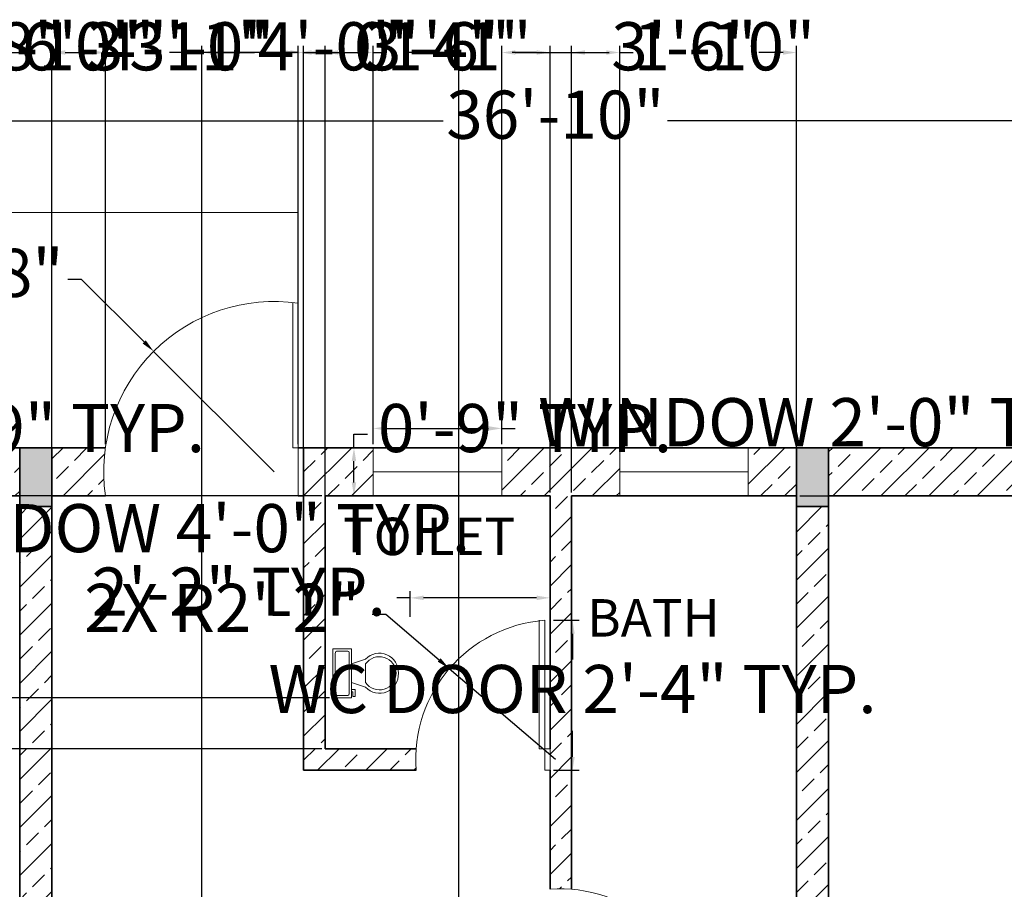
# Model space of a CAD drawing. Units: inches. Extents: x 9689 to 10369, y 10965 to 11626.
# Tile 8 of 11: x 9923 to 10107, y 11456 to 11619. Entities that reach past the tile are written whole.
import ezdxf

# ---------------------------------------------------------------- set-up
doc = ezdxf.new("R2010")
doc.units = ezdxf.units.IN
for name, color, linetype, lineweight in [('A-ANNO-DIMS', 2, 'Continuous', 18), ('A-AREA-IDEN', 7, 'Continuous', 18), ('A-COLS', 7, 'Continuous', 35), ('A-DOOR', 4, 'Continuous', 18), ('A-FLOR-FIXT', 8, 'Continuous', 18), ('A-FLOR-STRS', 7, 'Continuous', 18), ('A-GLAZ', 4, 'Continuous', 18), ('A-WALL', 7, 'Continuous', 35), ('A-WALL-PATT', 252, 'Continuous', 13)]:
    doc.layers.add(name, color=color, linetype=linetype, lineweight=lineweight)
doc.layers.add('A-COLS-PATT', color=18, linetype='Continuous', lineweight=13, true_color=0x000000)
doc.styles.get("Standard").update_dxf_attribs({"font": 'arial.ttf'})
doc.dimstyles.new('ISO-25', dxfattribs={"dimtxt": 9, "dimasz": 2.5, "dimexe": 1.25, "dimexo": 0.625, "dimgap": 2, "dimtad": 0, "dimtih": 1, "dimtoh": 1, "dimdec": 1, "dimlunit": 4, "dimtxsty": 'Standard', "dimcen": 2.5, "dimadec": 0, "dimazin": 0, "dimtfac": 0.5, "dimtdec": 1, "dimtmove": 0, "dimatfit": 3, "dimfxl": 1, "dimarcsym": 0})

# ---------------------------------------------------------------- blocks, each defined once
blk = doc.blocks.new('*U16')
for p, q in [((241.3, -152.4), (241.3, -50.8)), ((-203.2, -215.9), (-203.2, -203.2)), ((-177.8, -203.2), (-177.8, -241.3)), ((-101.6, -203.2), (-152.4, -355.6)), ((101.6, -203.2), (152.4, -355.6)), ((-254, -215.9), (-203.2, -215.9)), ((-254, -241.3), (-254, -215.9)), ((-177.8, -241.3), (-254, -241.3)), ((101.6, -355.6), (-101.6, -355.6))]:
    blk.add_line(p, q)
blk.add_lwpolyline([(266.7, -203.2), (266.7, 0), (-266.7, 0), (-266.7, -203.2)], close=True)
for points in [[(-241.3, -50.8), (-241.3, -152.4)], [(215.9, -25.4), (-215.9, -25.4)], [(-215.9, -177.8), (215.9, -177.8)]]:
    blk.add_lwpolyline(points)
for centre, radius, start, end in [((-219.075, -47.625), 22.45064, 81.8699, 188.1301), ((219.075, -47.625), 22.45064, 351.8699, 98.1301), ((-219.075, -155.575), 22.45064, 171.869898, 278.1301), ((219.075, -155.575), 22.45064, 261.8699, 8.1301), ((-12.12088, -505.93752), 205.61935, 133.01722, 273.38), ((0.94996, -504.77674), 181.02486, 124.50543, 269.7), ((-0.94742, -504.77674), 181.02486, 270.3, 55.4946), ((12.12342, -505.93752), 205.61935, 266.62, 46.9828)]:
    blk.add_arc(centre, radius, start, end)
blk = doc.blocks.new('*D21')
at = {"layer": 'A-ANNO-DIMS', "color": 0, "lineweight": -2, "transparency": 16777216}
for p, q in [((9802.06, 11539.26), (9802.06, 11600.92)), ((10244.06, 11539.26), (10244.06, 11600.92)), ((9804.56, 11599.67), (10002.11, 11599.67)), ((10241.56, 11599.67), (10044.01, 11599.67))]:
    blk.add_line(p, q, dxfattribs=at)
at = {"layer": 'A-ANNO-DIMS', "color": 0, "transparency": 16777216}
for points in [[(9804.56, 11600.08), (9804.56, 11599.25), (9802.06, 11599.67)], [(10241.56, 11600.08), (10241.56, 11599.25), (10244.06, 11599.67)]]:
    blk.add_solid(points, dxfattribs=at)
at = {"layer": 'Defpoints', "color": 0, "transparency": 16777216}
for p in [(10244.06, 11599.67), (9802.06, 11538.63), (10244.06, 11538.63)]:
    blk.add_point(p, dxfattribs=at)
at = {"layer": 'A-ANNO-DIMS', "color": 0, "transparency": 16777216, "insert": (10023.06, 11599.67), "char_height": 9, "attachment_point": 5}
blk.add_mtext('36\'-10"', dxfattribs=at)
blk = doc.blocks.new('WINDOW-24')
for p, q in [((0, 0), (0, 9)), ((24, 0), (24, 9)), ((0, 4.5), (24, 4.5))]:
    blk.add_line(p, q)
blk = doc.blocks.new('DOOR-SWING-24')
for p, q in [((4, 2), (28, 2)), ((4, 2), (4, 0)), ((0, 1), (4, 1)), ((0, 1), (0, 0)), ((0, 0), (4, 0)), ((4, 1), (28, 1))]:
    blk.add_line(p, q)
blk.add_arc((2, -1), 26.08, 4.3987, 94.3987)
blk = doc.blocks.new('*D34')
at = {"layer": 'A-ANNO-DIMS', "color": 0, "lineweight": -2, "transparency": 16777216}
for p, q in [((10022.68, 11506.38), (10027.51, 11506.38)), ((10026.26, 11503.88), (10026.26, 11499.04)), ((10026.26, 11480.88), (10026.26, 11485.72)), ((10022.68, 11478.38), (10027.51, 11478.38))]:
    blk.add_line(p, q, dxfattribs=at)
at = {"layer": 'A-ANNO-DIMS', "color": 0, "transparency": 16777216}
for points in [[(10025.84, 11503.88), (10026.67, 11503.88), (10026.26, 11506.38)], [(10025.84, 11480.88), (10026.67, 11480.88), (10026.26, 11478.38)]]:
    blk.add_solid(points, dxfattribs=at)
at = {"layer": 'Defpoints', "color": 0, "transparency": 16777216}
for p in [(10022.06, 11506.38), (10026.26, 11506.38), (10022.06, 11478.38)]:
    blk.add_point(p, dxfattribs=at)
at = {"layer": 'A-ANNO-DIMS', "color": 0, "transparency": 16777216, "insert": (10026.26, 11492.38), "char_height": 9, "attachment_point": 5}
blk.add_mtext('WC DOOR 2\'-4" TYP.', dxfattribs=at)
blk = doc.blocks.new('*D35')
at = {"layer": 'A-ANNO-DIMS', "color": 0, "lineweight": -2, "transparency": 16777216}
for p, q in [((9995.95, 11507.01), (9995.95, 11511.83)), ((10022.06, 11507.01), (10022.06, 11511.83)), ((9995.95, 11510.58), (9993.45, 11510.58)), ((10019.56, 11510.58), (9998.45, 11510.58))]:
    blk.add_line(p, q, dxfattribs=at)
at = {"layer": 'A-ANNO-DIMS', "color": 0, "transparency": 16777216}
for points in [[(9998.45, 11511), (9998.45, 11510.16), (9995.95, 11510.58)], [(10019.56, 11511), (10019.56, 11510.16), (10022.06, 11510.58)]]:
    blk.add_solid(points, dxfattribs=at)
at = {"layer": 'Defpoints', "color": 0, "transparency": 16777216}
for p in [(9995.95, 11510.58), (9995.95, 11506.38), (10022.06, 11506.38)]:
    blk.add_point(p, dxfattribs=at)
at = {"layer": 'A-ANNO-DIMS', "color": 0, "transparency": 16777216, "insert": (9963.95, 11510.58), "char_height": 9, "attachment_point": 5}
blk.add_mtext('2\'-2" TYP.', dxfattribs=at)
blk = doc.blocks.new('*D42')
at = {"layer": 'A-ANNO-DIMS', "color": 0, "lineweight": -2, "transparency": 16777216}
for p, q in [((9843.06, 11529.01), (9843.06, 11521.18)), ((9891.06, 11529.01), (9891.06, 11521.18)), ((9845.56, 11522.43), (9888.56, 11522.43)), ((9891.06, 11522.43), (9893.56, 11522.43))]:
    blk.add_line(p, q, dxfattribs=at)
at = {"layer": 'A-ANNO-DIMS', "color": 0, "transparency": 16777216}
for points in [[(9845.56, 11522.85), (9845.56, 11522.01), (9843.06, 11522.43)], [(9888.56, 11522.85), (9888.56, 11522.01), (9891.06, 11522.43)]]:
    blk.add_solid(points, dxfattribs=at)
at = {"layer": 'Defpoints', "color": 0, "transparency": 16777216}
for p in [(9843.06, 11529.63), (9891.06, 11529.63), (9891.06, 11522.43)]:
    blk.add_point(p, dxfattribs=at)
at = {"layer": 'A-ANNO-DIMS', "color": 0, "transparency": 16777216, "insert": (9952.5, 11522.43), "char_height": 9, "attachment_point": 5}
blk.add_mtext('WINDOW 4\'-0" TYP.', dxfattribs=at)
blk = doc.blocks.new('*D43')
at = {"layer": 'A-ANNO-DIMS', "color": 0, "lineweight": -2, "transparency": 16777216}
for p, q in [((9898.26, 11538.63), (9898.26, 11541.13)), ((9898.26, 11541.13), (9900.76, 11541.13)), ((9891.68, 11538.63), (9899.51, 11538.63)), ((9898.26, 11532.13), (9898.26, 11536.13)), ((9891.68, 11529.63), (9899.51, 11529.63))]:
    blk.add_line(p, q, dxfattribs=at)
at = {"layer": 'A-ANNO-DIMS', "color": 0, "transparency": 16777216}
for points in [[(9897.84, 11536.13), (9898.67, 11536.13), (9898.26, 11538.63)], [(9897.84, 11532.13), (9898.67, 11532.13), (9898.26, 11529.63)]]:
    blk.add_solid(points, dxfattribs=at)
at = {"layer": 'Defpoints', "color": 0, "transparency": 16777216}
for p in [(9891.06, 11538.63), (9898.26, 11538.63), (9891.06, 11529.63)]:
    blk.add_point(p, dxfattribs=at)
at = {"layer": 'A-ANNO-DIMS', "color": 0, "transparency": 16777216, "insert": (9930.19, 11541.13), "char_height": 9, "attachment_point": 5}
blk.add_mtext('0\'-9" TYP.', dxfattribs=at)
blk = doc.blocks.new('*D44')
at = {"layer": 'A-ANNO-DIMS', "color": 0, "lineweight": -2, "transparency": 16777216}
for p, q in [((9989.06, 11539.26), (9989.06, 11543.48)), ((10013.06, 11539.26), (10013.06, 11543.48)), ((9991.56, 11542.23), (10010.56, 11542.23)), ((10013.06, 11542.23), (10015.56, 11542.23))]:
    blk.add_line(p, q, dxfattribs=at)
at = {"layer": 'A-ANNO-DIMS', "color": 0, "transparency": 16777216}
for points in [[(9991.56, 11542.65), (9991.56, 11541.81), (9989.06, 11542.23)], [(10010.56, 11542.65), (10010.56, 11541.81), (10013.06, 11542.23)]]:
    blk.add_solid(points, dxfattribs=at)
at = {"layer": 'Defpoints', "color": 0, "transparency": 16777216}
for p in [(10013.06, 11542.23), (9989.06, 11538.63), (10013.06, 11538.63)]:
    blk.add_point(p, dxfattribs=at)
at = {"layer": 'A-ANNO-DIMS', "color": 0, "transparency": 16777216, "insert": (10074.5, 11542.23), "char_height": 9, "attachment_point": 5}
blk.add_mtext('WINDOW 2\'-0" TYP.', dxfattribs=at)
blk = doc.blocks.new('*D45')
at = {"layer": 'A-ANNO-DIMS', "color": 0, "lineweight": -2, "transparency": 16777216}
for p, q in [((9985.46, 11538.63), (9985.46, 11541.13)), ((9985.46, 11541.13), (9987.96, 11541.13)), ((9988.43, 11538.63), (9984.21, 11538.63)), ((9985.46, 11532.13), (9985.46, 11536.13)), ((9988.43, 11529.63), (9984.21, 11529.63))]:
    blk.add_line(p, q, dxfattribs=at)
at = {"layer": 'A-ANNO-DIMS', "color": 0, "transparency": 16777216}
for points in [[(9985.04, 11536.13), (9985.87, 11536.13), (9985.46, 11538.63)], [(9985.04, 11532.13), (9985.87, 11532.13), (9985.46, 11529.63)]]:
    blk.add_solid(points, dxfattribs=at)
at = {"layer": 'Defpoints', "color": 0, "transparency": 16777216}
for p in [(9985.46, 11538.63), (9989.06, 11538.63), (9989.06, 11529.63)]:
    blk.add_point(p, dxfattribs=at)
at = {"layer": 'A-ANNO-DIMS', "color": 0, "transparency": 16777216, "insert": (10017.39, 11541.13), "char_height": 9, "attachment_point": 5}
blk.add_mtext('0\'-9" TYP.', dxfattribs=at)
blk = doc.blocks.new('*D78')
at = {"layer": 'A-ANNO-DIMS', "color": 0, "lineweight": -2, "transparency": 16777216}
for p, q in [((9980.06, 11530.26), (9980.06, 11613.7)), ((10022.06, 11530.26), (10022.06, 11613.7)), ((9982.56, 11612.45), (9987.1, 11612.45)), ((10019.56, 11612.45), (10015.02, 11612.45))]:
    blk.add_line(p, q, dxfattribs=at)
at = {"layer": 'A-ANNO-DIMS', "color": 0, "transparency": 16777216}
for points in [[(9982.56, 11612.87), (9982.56, 11612.04), (9980.06, 11612.45)], [(10019.56, 11612.87), (10019.56, 11612.04), (10022.06, 11612.45)]]:
    blk.add_solid(points, dxfattribs=at)
at = {"layer": 'Defpoints', "color": 0, "transparency": 16777216}
for p in [(10022.06, 11612.45), (9980.06, 11529.63), (10022.06, 11529.63)]:
    blk.add_point(p, dxfattribs=at)
at = {"layer": 'A-ANNO-DIMS', "color": 0, "transparency": 16777216, "insert": (10001.06, 11612.45), "char_height": 9, "attachment_point": 5}
blk.add_mtext('3\'-6"', dxfattribs=at)
blk = doc.blocks.new('*D79')
at = {"layer": 'A-ANNO-DIMS', "color": 0, "lineweight": -2, "transparency": 16777216}
for p, q in [((10026.06, 11530.26), (10026.06, 11613.7)), ((10068.06, 11530.26), (10068.06, 11613.7)), ((10028.56, 11612.45), (10033.1, 11612.45)), ((10065.56, 11612.45), (10061.02, 11612.45))]:
    blk.add_line(p, q, dxfattribs=at)
at = {"layer": 'A-ANNO-DIMS', "color": 0, "transparency": 16777216}
for points in [[(10028.56, 11612.87), (10028.56, 11612.04), (10026.06, 11612.45)], [(10065.56, 11612.87), (10065.56, 11612.04), (10068.06, 11612.45)]]:
    blk.add_solid(points, dxfattribs=at)
at = {"layer": 'Defpoints', "color": 0, "transparency": 16777216}
for p in [(10068.06, 11612.45), (10026.06, 11529.63), (10068.06, 11529.63)]:
    blk.add_point(p, dxfattribs=at)
at = {"layer": 'A-ANNO-DIMS', "color": 0, "transparency": 16777216, "insert": (10047.06, 11612.45), "char_height": 9, "attachment_point": 5}
blk.add_mtext('3\'-6"', dxfattribs=at)
blk = doc.blocks.new('*D80')
at = {"layer": 'A-ANNO-DIMS', "color": 0, "lineweight": -2, "transparency": 16777216}
for p, q in [((9979.43, 11529.63), (9758.91, 11529.63)), ((9760.16, 11527.13), (9760.16, 11512.66)), ((9760.16, 11484.88), (9760.16, 11499.35)), ((9979.43, 11482.38), (9758.91, 11482.38))]:
    blk.add_line(p, q, dxfattribs=at)
at = {"layer": 'A-ANNO-DIMS', "color": 0, "transparency": 16777216}
for points in [[(9759.74, 11527.13), (9760.57, 11527.13), (9760.16, 11529.63)], [(9759.74, 11484.88), (9760.57, 11484.88), (9760.16, 11482.38)]]:
    blk.add_solid(points, dxfattribs=at)
at = {"layer": 'Defpoints', "color": 0, "transparency": 16777216}
for p in [(9760.16, 11529.63), (9980.06, 11529.63), (9980.06, 11482.38)]:
    blk.add_point(p, dxfattribs=at)
at = {"layer": 'A-ANNO-DIMS', "color": 0, "transparency": 16777216, "insert": (9760.16, 11506.01), "char_height": 9, "attachment_point": 5}
blk.add_mtext('3\'-11 1/2"', dxfattribs=at)
blk = doc.blocks.new('*D81')
at = {"layer": 'A-ANNO-DIMS', "color": 0, "lineweight": -2, "transparency": 16777216}
for p, q in [((10068.68, 11529.63), (10287.21, 11529.63)), ((10285.96, 11527.13), (10285.96, 11487.03)), ((10285.96, 11433.63), (10285.96, 11473.73)), ((10068.68, 11431.13), (10287.21, 11431.13))]:
    blk.add_line(p, q, dxfattribs=at)
at = {"layer": 'A-ANNO-DIMS', "color": 0, "transparency": 16777216}
for points in [[(10285.54, 11527.13), (10286.37, 11527.13), (10285.96, 11529.63)], [(10285.54, 11433.63), (10286.37, 11433.63), (10285.96, 11431.13)]]:
    blk.add_solid(points, dxfattribs=at)
at = {"layer": 'Defpoints', "color": 0, "transparency": 16777216}
for p in [(10068.06, 11529.63), (10285.96, 11529.63), (10068.06, 11431.13)]:
    blk.add_point(p, dxfattribs=at)
at = {"layer": 'A-ANNO-DIMS', "color": 0, "transparency": 16777216, "insert": (10285.96, 11480.38), "char_height": 9, "attachment_point": 5}
blk.add_mtext('8\'-2 1/2"', dxfattribs=at)
blk = doc.blocks.new('*D83')
at = {"layer": 'A-ANNO-DIMS', "color": 0, "lineweight": -2, "transparency": 16777216}
for p, q in [((9899.06, 11583.18), (9899.06, 11613.7)), ((9975.06, 11583.18), (9975.06, 11613.7)), ((9901.56, 11612.45), (9923.07, 11612.45)), ((9972.56, 11612.45), (9951.04, 11612.45))]:
    blk.add_line(p, q, dxfattribs=at)
at = {"layer": 'A-ANNO-DIMS', "color": 0, "transparency": 16777216}
for points in [[(9901.56, 11612.87), (9901.56, 11612.04), (9899.06, 11612.45)], [(9972.56, 11612.87), (9972.56, 11612.04), (9975.06, 11612.45)]]:
    blk.add_solid(points, dxfattribs=at)
at = {"layer": 'Defpoints', "color": 0, "transparency": 16777216}
for p in [(9975.06, 11612.45), (9899.06, 11582.55), (9975.06, 11582.55)]:
    blk.add_point(p, dxfattribs=at)
at = {"layer": 'A-ANNO-DIMS', "color": 0, "transparency": 16777216, "insert": (9937.06, 11612.45), "char_height": 9, "attachment_point": 5}
blk.add_mtext('6\'-4"', dxfattribs=at)
blk = doc.blocks.new('*D84')
at = {"layer": 'A-ANNO-DIMS', "color": 0, "lineweight": -2, "transparency": 16777216}
for p, q in [((9939.06, 11539.26), (9939.06, 11613.7)), ((9975.06, 11539.26), (9975.06, 11613.7)), ((9936.56, 11612.45), (9934.06, 11612.45)), ((9939.06, 11612.45), (9943.1, 11612.45)), ((9975.06, 11612.45), (9971.02, 11612.45)), ((9977.56, 11612.45), (9980.06, 11612.45))]:
    blk.add_line(p, q, dxfattribs=at)
at = {"layer": 'A-ANNO-DIMS', "color": 0, "transparency": 16777216}
for points in [[(9936.56, 11612.87), (9936.56, 11612.04), (9939.06, 11612.45)], [(9977.56, 11612.87), (9977.56, 11612.04), (9975.06, 11612.45)]]:
    blk.add_solid(points, dxfattribs=at)
at = {"layer": 'Defpoints', "color": 0, "transparency": 16777216}
for p in [(9975.06, 11612.45), (9939.06, 11538.63), (9975.06, 11538.63)]:
    blk.add_point(p, dxfattribs=at)
at = {"layer": 'A-ANNO-DIMS', "color": 0, "transparency": 16777216, "insert": (9957.06, 11612.45), "char_height": 9, "attachment_point": 5}
blk.add_mtext('3\'-0"', dxfattribs=at)
blk = doc.blocks.new('*D97')
at = {"layer": 'A-ANNO-DIMS', "color": 0, "lineweight": -2, "transparency": 16777216}
for p, q in [((9957.06, 11321.26), (9957.06, 11613.7)), ((10005.06, 11321.26), (10005.06, 11613.7)), ((9959.56, 11612.45), (9966.91, 11612.45)), ((10002.56, 11612.45), (9995.2, 11612.45))]:
    blk.add_line(p, q, dxfattribs=at)
at = {"layer": 'A-ANNO-DIMS', "color": 0, "transparency": 16777216}
for points in [[(9959.56, 11612.87), (9959.56, 11612.04), (9957.06, 11612.45)], [(10002.56, 11612.87), (10002.56, 11612.04), (10005.06, 11612.45)]]:
    blk.add_solid(points, dxfattribs=at)
at = {"layer": 'Defpoints', "color": 0, "transparency": 16777216}
for p in [(10005.06, 11612.45), (9957.06, 11320.63), (10005.06, 11320.63)]:
    blk.add_point(p, dxfattribs=at)
at = {"layer": 'A-ANNO-DIMS', "color": 0, "transparency": 16777216, "insert": (9981.06, 11612.45), "char_height": 9, "attachment_point": 5}
blk.add_mtext('4\'-0"', dxfattribs=at)
blk = doc.blocks.new('*D98')
at = {"layer": 'A-ANNO-DIMS', "color": 0, "lineweight": -2, "transparency": 16777216}
for p, q in [((9929.06, 11530.26), (9929.06, 11613.7)), ((9976.06, 11530.26), (9976.06, 11613.7)), ((9931.56, 11612.45), (9935.1, 11612.45)), ((9973.56, 11612.45), (9970.01, 11612.45))]:
    blk.add_line(p, q, dxfattribs=at)
at = {"layer": 'A-ANNO-DIMS', "color": 0, "transparency": 16777216}
for points in [[(9931.56, 11612.87), (9931.56, 11612.04), (9929.06, 11612.45)], [(9973.56, 11612.87), (9973.56, 11612.04), (9976.06, 11612.45)]]:
    blk.add_solid(points, dxfattribs=at)
at = {"layer": 'Defpoints', "color": 0, "transparency": 16777216}
for p in [(9976.06, 11612.45), (9929.06, 11529.63), (9976.06, 11529.63)]:
    blk.add_point(p, dxfattribs=at)
at = {"layer": 'A-ANNO-DIMS', "color": 0, "transparency": 16777216, "insert": (9952.56, 11612.45), "char_height": 9, "attachment_point": 5}
blk.add_mtext('3\'-11"', dxfattribs=at)
blk = doc.blocks.new('*D100')
at = {"layer": 'A-ANNO-DIMS', "color": 0, "lineweight": -2, "transparency": 16777216}
for p, q in [((10013.06, 11539.26), (10013.06, 11613.7)), ((10035.06, 11539.26), (10035.06, 11613.7)), ((10015.56, 11612.45), (10032.56, 11612.45)), ((10035.06, 11612.45), (10037.56, 11612.45))]:
    blk.add_line(p, q, dxfattribs=at)
at = {"layer": 'A-ANNO-DIMS', "color": 0, "transparency": 16777216}
for points in [[(10015.56, 11612.87), (10015.56, 11612.04), (10013.06, 11612.45)], [(10032.56, 11612.87), (10032.56, 11612.04), (10035.06, 11612.45)]]:
    blk.add_solid(points, dxfattribs=at)
at = {"layer": 'Defpoints', "color": 0, "transparency": 16777216}
for p in [(10035.06, 11612.45), (10013.06, 11538.63), (10035.06, 11538.63)]:
    blk.add_point(p, dxfattribs=at)
at = {"layer": 'A-ANNO-DIMS', "color": 0, "transparency": 16777216, "insert": (10054.59, 11612.45), "char_height": 9, "attachment_point": 5}
blk.add_mtext('1\'-10"', dxfattribs=at)
blk = doc.blocks.new('*D101')
at = {"layer": 'A-ANNO-DIMS', "color": 0, "lineweight": -2, "transparency": 16777216}
for p, q in [((9891.06, 11539.26), (9891.06, 11613.7)), ((9899.06, 11539.26), (9899.06, 11613.7)), ((9888.56, 11612.45), (9886.06, 11612.45)), ((9891.06, 11612.45), (9899.06, 11612.45)), ((9901.56, 11612.45), (9904.06, 11612.45))]:
    blk.add_line(p, q, dxfattribs=at)
at = {"layer": 'A-ANNO-DIMS', "color": 0, "transparency": 16777216}
for points in [[(9888.56, 11612.87), (9888.56, 11612.04), (9891.06, 11612.45)], [(9901.56, 11612.87), (9901.56, 11612.04), (9899.06, 11612.45)]]:
    blk.add_solid(points, dxfattribs=at)
at = {"layer": 'Defpoints', "color": 0, "transparency": 16777216}
for p in [(9899.06, 11612.45), (9891.06, 11538.63), (9899.06, 11538.63)]:
    blk.add_point(p, dxfattribs=at)
at = {"layer": 'A-ANNO-DIMS', "color": 0, "transparency": 16777216, "insert": (9918.02, 11612.45), "char_height": 9, "attachment_point": 5}
blk.add_mtext('0\'-8"', dxfattribs=at)
blk = doc.blocks.new('*D106')
at = {"layer": 'A-ANNO-DIMS', "color": 0, "lineweight": -2, "transparency": 16777216}
for p, q in [((9976.06, 11479.01), (9976.06, 11613.7)), ((9980.06, 11483.01), (9980.06, 11613.7)), ((9973.56, 11612.45), (9971.06, 11612.45)), ((9976.06, 11612.45), (9980.06, 11612.45)), ((9982.56, 11612.45), (9985.06, 11612.45))]:
    blk.add_line(p, q, dxfattribs=at)
at = {"layer": 'A-ANNO-DIMS', "color": 0, "transparency": 16777216}
for points in [[(9973.56, 11612.87), (9973.56, 11612.04), (9976.06, 11612.45)], [(9982.56, 11612.87), (9982.56, 11612.04), (9980.06, 11612.45)]]:
    blk.add_solid(points, dxfattribs=at)
at = {"layer": 'Defpoints', "color": 0, "transparency": 16777216}
for p in [(9980.06, 11612.45), (9980.06, 11482.38), (9976.06, 11478.38)]:
    blk.add_point(p, dxfattribs=at)
at = {"layer": 'A-ANNO-DIMS', "color": 0, "transparency": 16777216, "insert": (9999.02, 11612.45), "char_height": 9, "attachment_point": 5}
blk.add_mtext('0\'-4"', dxfattribs=at)
blk = doc.blocks.new('*D109')
at = {"layer": 'A-ANNO-DIMS', "color": 0, "lineweight": -2, "transparency": 16777216}
for p, q in [((9976.06, 11539.26), (9976.06, 11613.7)), ((9989.06, 11539.26), (9989.06, 11613.7)), ((9978.56, 11612.45), (9986.56, 11612.45)), ((9989.06, 11612.45), (9991.56, 11612.45))]:
    blk.add_line(p, q, dxfattribs=at)
at = {"layer": 'A-ANNO-DIMS', "color": 0, "transparency": 16777216}
for points in [[(9978.56, 11612.87), (9978.56, 11612.04), (9976.06, 11612.45)], [(9986.56, 11612.87), (9986.56, 11612.04), (9989.06, 11612.45)]]:
    blk.add_solid(points, dxfattribs=at)
at = {"layer": 'Defpoints', "color": 0, "transparency": 16777216}
for p in [(9989.06, 11612.45), (9976.06, 11538.63), (9989.06, 11538.63)]:
    blk.add_point(p, dxfattribs=at)
at = {"layer": 'A-ANNO-DIMS', "color": 0, "transparency": 16777216, "insert": (10005.1, 11612.45), "char_height": 9, "attachment_point": 5}
blk.add_mtext('1\'-1"', dxfattribs=at)
blk = doc.blocks.new('*D111')
at = {"layer": 'A-ANNO-DIMS', "color": 0, "lineweight": -2, "transparency": 16777216}
for p, q in [((9899.06, 11583.18), (9899.06, 11613.7)), ((9909.06, 11583.18), (9909.06, 11613.7)), ((9901.56, 11612.45), (9906.56, 11612.45)), ((9909.06, 11612.45), (9911.56, 11612.45))]:
    blk.add_line(p, q, dxfattribs=at)
at = {"layer": 'A-ANNO-DIMS', "color": 0, "transparency": 16777216}
for points in [[(9901.56, 11612.87), (9901.56, 11612.04), (9899.06, 11612.45)], [(9906.56, 11612.87), (9906.56, 11612.04), (9909.06, 11612.45)]]:
    blk.add_solid(points, dxfattribs=at)
at = {"layer": 'Defpoints', "color": 0, "transparency": 16777216}
for p in [(9909.06, 11612.45), (9899.06, 11582.55), (9909.06, 11582.55)]:
    blk.add_point(p, dxfattribs=at)
at = {"layer": 'A-ANNO-DIMS', "color": 0, "transparency": 16777216, "insert": (9929.02, 11612.45), "char_height": 9, "attachment_point": 5}
blk.add_mtext('0\'-10"', dxfattribs=at)
blk = doc.blocks.new('*D118')
at = {"layer": 'A-ANNO-DIMS', "color": 0, "lineweight": -2, "transparency": 16777216}
for p, q in [((9980.91, 11491.91), (9758.91, 11491.91)), ((9760.16, 11489.41), (9760.16, 11484.88)), ((9979.43, 11482.38), (9758.91, 11482.38)), ((9760.16, 11482.38), (9760.16, 11479.88)), ((9760.16, 11479.88), (9757.66, 11479.88))]:
    blk.add_line(p, q, dxfattribs=at)
at = {"layer": 'A-ANNO-DIMS', "color": 0, "transparency": 16777216}
for points in [[(9759.74, 11489.41), (9760.57, 11489.41), (9760.16, 11491.91)], [(9759.74, 11484.88), (9760.57, 11484.88), (9760.16, 11482.38)]]:
    blk.add_solid(points, dxfattribs=at)
at = {"layer": 'Defpoints', "color": 0, "transparency": 16777216}
for p in [(9981.53, 11491.91), (9760.16, 11482.38), (9980.06, 11482.38)]:
    blk.add_point(p, dxfattribs=at)
at = {"layer": 'A-ANNO-DIMS', "color": 0, "transparency": 16777216, "insert": (9733.21, 11479.88), "char_height": 9, "attachment_point": 5}
blk.add_mtext('0\'-9 1/2"', dxfattribs=at)
blk = doc.blocks.new('*D120')
at = {"layer": 'A-ANNO-DIMS', "color": 0, "lineweight": -2, "transparency": 16777216}
for p, q in [((9932.06, 11570.13), (9934.56, 11570.13)), ((9934.56, 11570.13), (9946.29, 11558.4)), ((9970.56, 11534.13), (9948.06, 11556.63))]:
    blk.add_line(p, q, dxfattribs=at)
at = {"layer": 'A-ANNO-DIMS', "color": 0, "transparency": 16777216}
blk.add_solid([(9946.58, 11558.69), (9945.99, 11558.1), (9948.06, 11556.63)], dxfattribs=at)
at = {"layer": 'Defpoints', "color": 0, "transparency": 16777216}
for p in [(9948.06, 11556.63), (9970.56, 11534.13)]:
    blk.add_point(p, dxfattribs=at)
at = {"layer": 'A-ANNO-DIMS', "color": 0, "transparency": 16777216, "insert": (9913.79, 11570.13), "char_height": 9, "attachment_point": 5}
blk.add_mtext('R2\'-8"', dxfattribs=at)
blk = doc.blocks.new('*D122')
at = {"layer": 'A-ANNO-DIMS', "color": 0, "lineweight": -2, "transparency": 16777216}
for p, q in [((9988.88, 11507.53), (9991.38, 11507.53)), ((9991.38, 11507.53), (10001.36, 11498.98)), ((10023.06, 11480.38), (10003.26, 11497.35))]:
    blk.add_line(p, q, dxfattribs=at)
at = {"layer": 'A-ANNO-DIMS', "color": 0, "transparency": 16777216}
blk.add_solid([(10001.63, 11499.29), (10001.09, 11498.66), (10003.26, 11497.35)], dxfattribs=at)
at = {"layer": 'Defpoints', "color": 0, "transparency": 16777216}
for p in [(10003.26, 11497.35), (10023.06, 11480.38)]:
    blk.add_point(p, dxfattribs=at)
at = {"layer": 'A-ANNO-DIMS', "color": 0, "transparency": 16777216, "insert": (9960.86, 11507.53), "char_height": 9, "attachment_point": 5}
blk.add_mtext('2X R2\'-2"', dxfattribs=at)

msp = doc.modelspace()

# ---------------------------------------------------------------- hatches: boundary and pattern name
at = {"layer": 'A-COLS-PATT'}
h = msp.add_hatch(color=256, dxfattribs=at)
h.dxf.hatch_style = 1
h.paths.add_polyline_path([(9929.06, 11538.63), (9923.06, 11538.63), (9923.06, 11529.63), (9923.06, 11527.63), (9929.06, 11527.63), (9929.06, 11529.63)])
h = msp.add_hatch(color=256, dxfattribs=at)
h.dxf.hatch_style = 1
h.paths.add_polyline_path([(10074.06, 11538.63), (10068.06, 11538.63), (10068.06, 11529.63), (10068.06, 11527.63), (10074.06, 11527.63), (10074.06, 11529.63)])
at = {"layer": 'A-WALL-PATT'}
h = msp.add_hatch(dxfattribs=at)
h.set_pattern_fill('ANSI33', color=256)
h.paths.add_polyline_path([(9843.06, 11538.63), (9811.06, 11538.63), (9811.06, 11529.63), (9843.06, 11529.63)])
h.paths.add_polyline_path([(9923.06, 11538.63), (9891.06, 11538.63), (9891.06, 11529.63), (9923.06, 11529.63)])
h.paths.add_polyline_path([(9929.06, 11527.63), (9923.06, 11527.63), (9923.06, 11380.63), (9929.06, 11380.63)])
h.paths.add_polyline_path([(9939.06, 11538.63), (9929.06, 11538.63), (9929.06, 11529.63), (9939.06, 11529.63, -0.071068)])
h.paths.add_polyline_path([(10035.06, 11538.63), (10013.06, 11538.63), (10013.06, 11529.63), (10022.06, 11529.63), (10022.06, 11507.38), (10022.06, 11502.38), (10022.06, 11482.38), (10022.06, 11478.38), (10022.06, 11456.13, -0.038405), (10026.06, 11456.13), (10026.06, 11502.38), (10026.06, 11529.63), (10035.06, 11529.63)])
h.paths.add_polyline_path([(10068.06, 11538.63), (10059.06, 11538.63), (10059.06, 11529.63), (10068.06, 11529.63)])
h.paths.add_polyline_path([(10074.06, 11527.63), (10068.06, 11527.63), (10068.06, 11431.13), (10026.06, 11431.13), (10022.06, 11431.13), (9980.06, 11431.13), (9976.06, 11431.13), (9976.06, 11425.13), (10068.06, 11425.13), (10068.06, 11380.63), (10074.06, 11380.63)])
h.paths.add_polyline_path([(10124.56, 11538.63), (10074.06, 11538.63), (10074.06, 11529.63), (10124.56, 11529.63)])
h.paths.add_polyline_path([(9980.06, 11507.38), (9980.06, 11529.63), (9989.06, 11529.63), (9989.06, 11538.63), (9976.06, 11538.63), (9976.06, 11529.63), (9976.06, 11503.38), (9976.06, 11483.38), (9976.06, 11478.38), (9980.06, 11478.38), (9997.06, 11478.38, -0.038405), (9997.06, 11482.38), (9980.06, 11482.38)])
h.paths.add_polyline_path([(10235.06, 11538.63), (10184.56, 11538.63), (10184.56, 11529.63), (10235.06, 11529.63)])
h.paths.add_polyline_path([(10244.06, 11527.63), (10235.06, 11527.63), (10235.06, 11485.13), (10244.06, 11485.13)])
h.paths.add_polyline_path([(10244.06, 11425.13), (10235.06, 11425.13), (10235.06, 11380.63), (10244.06, 11380.63)])
h.paths.add_polyline_path([(10233.06, 11380.63), (10120.06, 11380.63, -0.038405), (10120.06, 11374.63), (10133.04, 11374.63), (10133.04, 11326.63), (10120.06, 11326.63, -0.038405), (10120.06, 11320.63), (10149.19, 11320.63), (10149.19, 11326.63), (10136.04, 11326.63), (10136.04, 11374.63), (10233.06, 11374.63)])
h.paths.add_polyline_path([(10084.06, 11380.63), (10076.06, 11380.63), (10076.06, 11374.63), (10084.06, 11374.63)])
h.paths.add_polyline_path([(10244.06, 11374.63), (10235.06, 11374.63), (10235.06, 11362.63), (10244.06, 11362.63)])
h.paths.add_polyline_path([(10244.06, 11338.63), (10235.06, 11338.63), (10235.06, 11326.63), (10244.06, 11326.63)])
h.paths.add_polyline_path([(10233.06, 11326.63), (10173.19, 11326.63, -0.055385), (10173.19, 11320.63), (10233.06, 11320.63)], flags=0)
h.paths.add_polyline_path([(10244.06, 11320.63), (10235.06, 11320.63), (10235.06, 11273.63), (10244.06, 11273.63)])
h = msp.add_hatch(dxfattribs=at)
h.set_pattern_fill('ANSI36', color=256)
h.paths.add_polyline_path([(10233.06, 11326.63), (10173.19, 11326.63, -0.055385), (10173.19, 11320.63), (10233.06, 11320.63)])
h.paths.add_polyline_path([(10244.06, 11213.63), (10235.06, 11213.63), (10235.06, 11166.63), (10244.06, 11166.63)])
h.paths.add_polyline_path([(10233.06, 11166.63), (10184.56, 11166.63), (10184.56, 11157.63), (10233.06, 11157.63)])
h.paths.add_polyline_path([(10124.56, 11166.63), (10074.06, 11166.63), (10074.06, 11157.63), (10124.56, 11157.63)])
h.paths.add_polyline_path([(10074.06, 11318.63), (10068.06, 11318.63), (10068.06, 11168.63), (10074.06, 11168.63)])
h.paths.add_polyline_path([(10068.06, 11166.63), (10011.06, 11166.63), (10011.06, 11157.63), (10068.06, 11157.63)])
h.paths.add_polyline_path([(10011.06, 11318.63), (10005.06, 11318.63), (10005.06, 11168.63), (10011.06, 11168.63)])
h.paths.add_polyline_path([(10005.06, 11166.63), (9985.06, 11166.63), (9985.06, 11157.63), (10005.06, 11157.63)])
h.paths.add_polyline_path([(9937.06, 11166.63), (9898.06, 11166.63), (9898.06, 11157.63), (9937.06, 11157.63, -0.042779)])
h.paths.add_polyline_path([(9850.06, 11166.63), (9813.06, 11166.63), (9813.06, 11157.63), (9850.06, 11157.63)])
h.paths.add_polyline_path([(9811.06, 11213.63), (9802.06, 11213.63), (9802.06, 11166.63), (9811.06, 11166.63)])
h.paths.add_polyline_path([(9811.06, 11320.63), (9802.06, 11320.63), (9802.06, 11273.63), (9811.06, 11273.63)])
h.paths.add_polyline_path([(9811.06, 11439.11), (9802.06, 11439.11), (9802.06, 11326.63), (9811.06, 11326.63)])
h.paths.add_polyline_path([(9957.06, 11326.63), (9813.06, 11326.63), (9813.06, 11320.63), (9957.06, 11320.63)])
h.paths.add_polyline_path([(9811.06, 11527.63), (9802.06, 11527.63), (9802.06, 11499.11), (9811.06, 11499.11)])

# ---------------------------------------------------------------- linework, layer by layer
at = {"layer": 'A-COLS'}
for p, q in [((9923.06, 11529.63), (9923.06, 11538.63)), ((9929.06, 11529.63), (9929.06, 11538.63)), ((10068.06, 11529.63), (10068.06, 11538.63)), ((10074.06, 11529.63), (10074.06, 11538.63)), ((9923.06, 11527.63), (9929.06, 11527.63)), ((10074.06, 11527.63), (10068.06, 11527.63))]:
    msp.add_line(p, q, dxfattribs=at)
at = {"layer": 'A-DOOR'}
for p, q in [((9974.06, 11538.63), (9974.06, 11565.63)), ((9975.06, 11529.63), (9975.06, 11565.63)), ((9975.06, 11538.63), (9974.06, 11538.63)), ((9975.06, 11529.63), (9975.06, 11538.63)), ((9975.06, 11538.63), (9975.06, 11529.63))]:
    msp.add_line(p, q, dxfattribs=at)
msp.add_arc((9970.56, 11534.13), 31.82, 81.8699, 188.1301, dxfattribs=at)
at = {"layer": 'A-FLOR-STRS'}
for p, q in [((9899.06, 11582.55), (9929.06, 11582.55)), ((9929.06, 11538.63), (9929.06, 11582.55)), ((9929.06, 11582.55), (9975.06, 11582.55)), ((9975.06, 11565.63), (9975.06, 11582.55))]:
    msp.add_line(p, q, dxfattribs=at)
at = {"layer": 'A-WALL'}
for p, q in [((9802.06, 11538.63), (9939.06, 11538.63)), ((9975.06, 11538.63), (10244.06, 11538.63)), ((9976.06, 11538.63), (9976.06, 11529.63)), ((9811.06, 11529.63), (9923.06, 11529.63)), ((9923.06, 11374.63), (9923.06, 11529.63)), ((9929.06, 11380.63), (9929.06, 11529.63)), ((9929.06, 11529.63), (9939.06, 11529.63)), ((9929.06, 11431.13), (9929.06, 11529.63)), ((9975.06, 11529.63), (9976.06, 11529.63)), ((9976.06, 11529.63), (9976.06, 11503.38)), ((9980.06, 11529.63), (9980.06, 11507.38)), ((9980.06, 11529.63), (10022.06, 11529.63)), ((10022.06, 11529.63), (10022.06, 11507.38)), ((10026.06, 11529.63), (10026.06, 11502.38)), ((10026.06, 11529.63), (10068.06, 11529.63)), ((10068.06, 11529.63), (10068.06, 11431.13)), ((10074.06, 11529.63), (10074.06, 11380.63)), ((10074.06, 11529.63), (10235.06, 11529.63)), ((9980.06, 11507.38), (9980.06, 11482.38)), ((10022.06, 11507.38), (10022.06, 11502.38)), ((9976.06, 11483.38), (9976.06, 11503.38)), ((10022.06, 11503.38), (10022.06, 11502.38)), ((10022.06, 11502.88), (10022.06, 11482.38)), ((10026.06, 11502.38), (10026.06, 11456.13)), ((9976.06, 11483.38), (9976.06, 11478.38)), ((9997.06, 11482.38), (9980.06, 11482.38)), ((9980.06, 11478.38), (9976.06, 11478.38)), ((9997.06, 11478.38), (9980.06, 11478.38)), ((10022.06, 11478.38), (10022.06, 11456.13))]:
    msp.add_line(p, q, dxfattribs=at)

# ---------------------------------------------------------------- block references
at = {"layer": 'A-DOOR', "rotation": 90.0000000000178}
msp.add_blockref('DOOR-SWING-24', (10022.06, 11478.38), dxfattribs=at)
at = {"layer": 'A-DOOR'}
msp.add_blockref('DOOR-SWING-24', (10022.06, 11431.13), dxfattribs=at)
at = {"layer": 'A-FLOR-FIXT', "xscale": 0.0171838114023506, "yscale": 0.0171838114023506, "zscale": 0.0171838114023506, "rotation": 90}
msp.add_blockref('*U16', (9981.53, 11496.49), dxfattribs=at)
at = {"layer": 'A-GLAZ'}
msp.add_blockref('WINDOW-24', (9989.06, 11529.63), dxfattribs=at)
at = {"layer": 'A-GLAZ', "rotation": 180}
msp.add_blockref('WINDOW-24', (10059.06, 11538.63), dxfattribs=at)

# ---------------------------------------------------------------- texts
at = {"layer": 'A-AREA-IDEN', "char_height": 7, "attachment_point": 1}
for s, width, insert in [('{\\fArial|b1|i0|c0|p34;TOILET}', 36.036, (9983.42, 11525.56)), ('{\\fArial|b1|i0|c0|p34;BATH}', 36.502, (10028.98, 11510.34))]:
    msp.add_mtext_dynamic_manual_height_columns(s, width=width, gutter_width=12.5, heights=[0], dxfattribs=dict(at, insert=insert))

# ---------------------------------------------------------------- dimensions: what is measured, and where the dimension line sits
at = {"layer": 'A-ANNO-DIMS'}
for base, p1, p2, override, picture, middle in [((9899.06, 11612.45), (9891.06, 11538.63), (9899.06, 11538.63), {"dimdec": 1, "dimlfac": 1, "dimrnd": 0, "dimzin": 1, "dimdsep": 46, "dimlunit": 4, "dimfrac": 2}, '*D101', (9918.02, 11612.45)), ((9975.06, 11612.45), (9899.06, 11582.55), (9975.06, 11582.55), {"dimdec": 1, "dimlfac": 1, "dimrnd": 0, "dimzin": 1, "dimdsep": 46, "dimlunit": 4, "dimfrac": 2}, '*D83', (9937.06, 11612.45)), ((9909.06, 11612.45), (9899.06, 11582.55), (9909.06, 11582.55), {"dimdec": 1, "dimlfac": 1, "dimrnd": 0, "dimzin": 1, "dimdsep": 46, "dimlunit": 4, "dimfrac": 2}, '*D111', (9929.02, 11612.45)), ((9976.06, 11612.45), (9929.06, 11529.63), (9976.06, 11529.63), {"dimdec": 1, "dimlfac": 1, "dimrnd": 0, "dimzin": 1, "dimdsep": 46, "dimlunit": 4, "dimfrac": 2}, '*D98', (9952.56, 11612.45)), ((9975.06, 11612.45), (9939.06, 11538.63), (9975.06, 11538.63), {"dimdec": 1, "dimlfac": 1, "dimrnd": 0, "dimzin": 1, "dimdsep": 46, "dimlunit": 4, "dimfrac": 2}, '*D84', (9957.06, 11612.45)), ((10005.06, 11612.45), (9957.06, 11320.63), (10005.06, 11320.63), {"dimdec": 1, "dimlfac": 1, "dimrnd": 0, "dimzin": 1, "dimdsep": 46, "dimlunit": 4, "dimfrac": 2}, '*D97', (9981.06, 11612.45)), ((9980.06, 11612.45), (9976.06, 11478.38), (9980.06, 11482.38), {"dimdec": 1, "dimlfac": 1, "dimrnd": 0, "dimzin": 1, "dimdsep": 46, "dimlunit": 4, "dimfrac": 2}, '*D106', (9999.02, 11612.45)), ((9989.06, 11612.45), (9976.06, 11538.63), (9989.06, 11538.63), {"dimdec": 1, "dimlfac": 1, "dimrnd": 0, "dimzin": 1, "dimdsep": 46, "dimlunit": 4, "dimfrac": 2}, '*D109', (10005.1, 11612.45)), ((10022.06, 11612.45), (9980.06, 11529.63), (10022.06, 11529.63), {"dimdec": 1, "dimlfac": 1, "dimrnd": 0, "dimzin": 1, "dimdsep": 46, "dimlunit": 4, "dimfrac": 2}, '*D78', (10001.06, 11612.45)), ((10035.06, 11612.45), (10013.06, 11538.63), (10035.06, 11538.63), {"dimdec": 1, "dimlfac": 1, "dimrnd": 0, "dimzin": 1, "dimdsep": 46, "dimlunit": 4, "dimfrac": 2}, '*D100', (10054.59, 11612.45)), ((10068.06, 11612.45), (10026.06, 11529.63), (10068.06, 11529.63), {"dimdec": 1, "dimlfac": 1, "dimrnd": 0, "dimzin": 1, "dimdsep": 46, "dimlunit": 4, "dimfrac": 2}, '*D79', (10047.06, 11612.45)), ((10244.06, 11599.67), (9802.06, 11538.63), (10244.06, 11538.63), {"dimclrd": 0, "dimclre": 0, "dimclrt": 0}, '*D21', (10023.06, 11599.67))]:
    dim = msp.add_linear_dim(base=base, p1=p1, p2=p2, dimstyle='ISO-25', override=override, dxfattribs=at)
    dim.commit()
    dim.dimension.update_dxf_attribs({"geometry": picture, "text_midpoint": middle})
dim = msp.add_radius_dim(center=(9970.56, 11534.13), mpoint=(9948.06, 11556.63), dimstyle='ISO-25', override={"dimdec": 1, "dimlfac": 1, "dimrnd": 0, "dimzin": 1, "dimdsep": 46, "dimlunit": 4, "dimfrac": 2}, dxfattribs=at)
dim.commit()
dim.dimension.update_dxf_attribs({"geometry": '*D120', "text_midpoint": (9913.79, 11570.13), "dimtype": 164})
for base, p1, p2, picture, middle in [((10013.06, 11542.23), (9989.06, 11538.63), (10013.06, 11538.63), '*D44', (10074.5, 11542.23)), ((9891.06, 11522.43), (9843.06, 11529.63), (9891.06, 11529.63), '*D42', (9952.5, 11522.43))]:
    dim = msp.add_linear_dim(base=base, p1=p1, p2=p2, text='WINDOW <> TYP.', dimstyle='ISO-25', override={"dimdec": 1, "dimlfac": 1, "dimrnd": 0, "dimzin": 1, "dimdsep": 46, "dimlunit": 4, "dimfrac": 2}, dxfattribs=at)
    dim.commit()
    dim.dimension.update_dxf_attribs({"geometry": picture, "text_midpoint": middle})
for base, p1, p2, angle, text, picture, middle in [((9898.26, 11538.63), (9891.06, 11529.63), (9891.06, 11538.63), 90, '<> TYP.', '*D43', (9930.19, 11541.13)), ((9985.46, 11538.63), (9989.06, 11529.63), (9989.06, 11538.63), 90, '<> TYP.', '*D45', (10017.39, 11541.13)), ((9995.95, 11510.58), (10022.06, 11506.38), (9995.95, 11506.38), 180, '<> TYP.', '*D35', (9963.95, 11510.58)), ((10026.26, 11506.38), (10022.06, 11478.38), (10022.06, 11506.38), 90, 'WC DOOR <> TYP.', '*D34', (10026.26, 11492.38))]:
    dim = msp.add_linear_dim(base=base, p1=p1, p2=p2, angle=angle, text=text, dimstyle='ISO-25', override={"dimdec": 1, "dimlfac": 1, "dimrnd": 0, "dimzin": 1, "dimdsep": 46, "dimlunit": 4, "dimfrac": 2}, dxfattribs=at)
    dim.commit()
    dim.dimension.update_dxf_attribs({"geometry": picture, "text_midpoint": middle})
for base, p1, p2, picture, middle in [((9760.15676, 11529.630116), (9980.05676, 11482.380116), (9980.05676, 11529.630116), '*D80', (9760.15676, 11506.005116)), ((10285.96, 11529.63), (10068.06, 11431.13), (10068.06, 11529.63), '*D81', (10285.96, 11480.38)), ((9760.16, 11482.38), (9981.53, 11491.91), (9980.06, 11482.38), '*D118', (9733.21, 11479.88))]:
    dim = msp.add_linear_dim(base=base, p1=p1, p2=p2, angle=90, dimstyle='ISO-25', override={"dimdec": 1, "dimlfac": 1, "dimrnd": 0, "dimzin": 1, "dimdsep": 46, "dimlunit": 4, "dimfrac": 2}, dxfattribs=at)
    dim.commit()
    dim.dimension.update_dxf_attribs({"geometry": picture, "text_midpoint": middle})
dim = msp.add_radius_dim(center=(10023.06, 11480.38), mpoint=(10003.26, 11497.35), text='2X <>', dimstyle='ISO-25', override={"dimdec": 1, "dimlfac": 1, "dimrnd": 0, "dimzin": 1, "dimdsep": 46, "dimlunit": 4, "dimfrac": 2}, dxfattribs=at)
dim.commit()
dim.dimension.update_dxf_attribs({"geometry": '*D122', "text_midpoint": (9960.86, 11507.53), "dimtype": 164})

doc.saveas('drawing.dxf')
